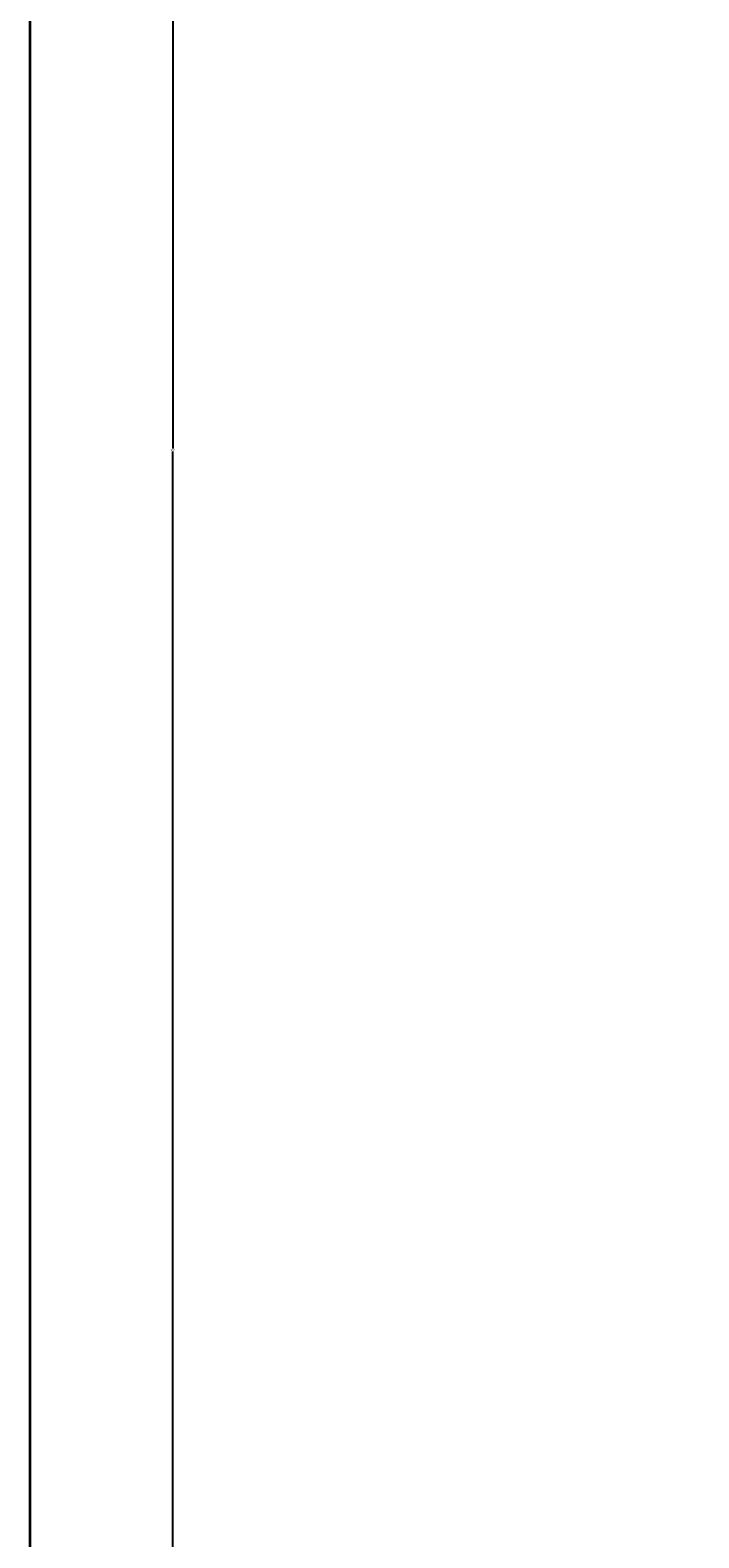
# Model space of a CAD drawing. Units: inches. Extents: x 1885 to 2748, y 783 to 2421.
# Tile 65 of 117: x 1885 to 1969, y 1979 to 2167. Entities that reach past the tile are written whole.
import ezdxf

# ---------------------------------------------------------------- set-up
doc = ezdxf.new("R2010")
doc.units = ezdxf.units.IN
doc.layers.add('A-ANNO-DIMS', color=2, linetype='Continuous', lineweight=18)
doc.layers.add('A-ANNO-TTLB', color=7, linetype='Continuous', lineweight=35)
doc.styles.get("Standard").update_dxf_attribs({"font": 'arial.ttf'})
doc.dimstyles.get("Standard").update_dxf_attribs({"dimtxt": 0.18, "dimasz": 0.18, "dimexe": 0.18, "dimexo": 0.0625, "dimgap": 0.09, "dimtad": 0, "dimtih": 1, "dimtoh": 1, "dimdec": 4, "dimzin": 0, "dimdsep": 46, "dimtxsty": 'Standard', "dimcen": 0.09, "dimadec": 0, "dimazin": 0, "dimtfac": 1, "dimtdec": 4, "dimtofl": 0, "dimtmove": 0, "dimatfit": 3, "dimfxl": 1, "dimtolj": 1, "dimtzin": 0, "dimarcsym": 0})

# ---------------------------------------------------------------- blocks, each defined once
blk = doc.blocks.new('*D48')
at = {"layer": 'A-ANNO-DIMS', "color": 0, "lineweight": -2, "transparency": 16777216}
for p, q in [((1980.71, 2348.01), (1902.84, 2348.01)), ((1903.02, 2347.83), (1903.02, 2114.94)), ((1903.02, 1881.69), (1903.02, 2114.57)), ((2016.71, 1881.51), (1902.84, 1881.51))]:
    blk.add_line(p, q, dxfattribs=at)
at = {"layer": 'A-ANNO-DIMS', "color": 0, "transparency": 16777216}
for points in [[(1902.99, 2347.83), (1903.05, 2347.83), (1903.02, 2348.01)], [(1902.99, 1881.69), (1903.05, 1881.69), (1903.02, 1881.51)]]:
    blk.add_solid(points, dxfattribs=at)
at = {"layer": 'Defpoints', "color": 0, "transparency": 16777216}
for p in [(1903.02, 2348.01), (1980.77, 2348.01), (2016.77, 1881.51)]:
    blk.add_point(p, dxfattribs=at)
at = {"layer": 'A-ANNO-DIMS', "color": 0, "transparency": 16777216, "insert": (1903.02, 2114.76), "char_height": 0.18, "attachment_point": 5}
blk.add_mtext('\\A1;466.5', dxfattribs=at)

msp = doc.modelspace()

# ---------------------------------------------------------------- linework, layer by layer
at = {"layer": 'A-ANNO-TTLB'}
msp.add_lwpolyline([(1885.16, 2409.17), (2748.2, 2409.17), (2748.2, 922.58), (1885.16, 922.58)], close=True, dxfattribs=at)

# ---------------------------------------------------------------- dimensions: what is measured, and where the dimension line sits
at = {"layer": 'A-ANNO-DIMS'}
dim = msp.add_linear_dim(base=(1903.02, 2348.01), p1=(2016.77, 1881.51), p2=(1980.77, 2348.01), angle=90, dimstyle='Standard', override={"dimdec": 1, "dimlfac": 1, "dimrnd": 0, "dimzin": 0, "dimdsep": 46, "dimlunit": 2}, dxfattribs=at)
dim.commit()
dim.dimension.update_dxf_attribs({"geometry": '*D48', "text_midpoint": (1903.02, 2114.76)})

doc.saveas('drawing.dxf')
